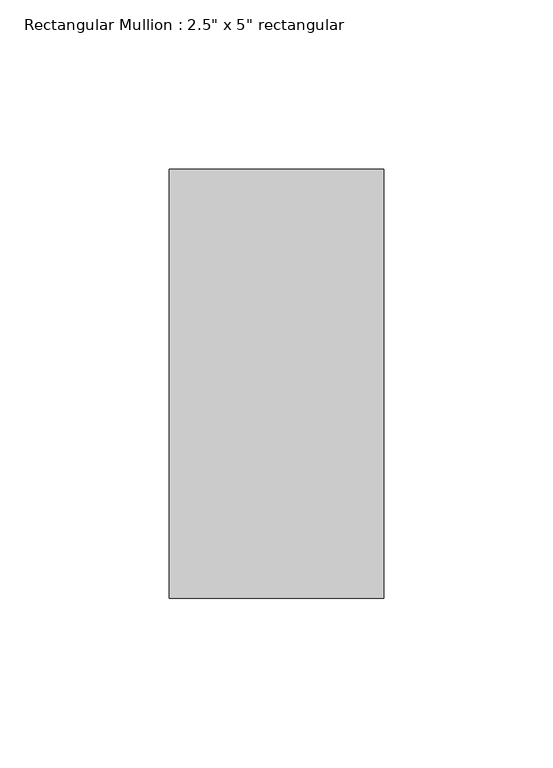
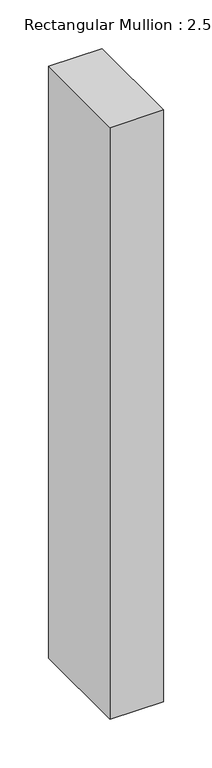
"""IFC4 building model written with IfcOpenShell, lengths in millimetres: member geometry."""

from ifc_helpers import new_model, si_unit, frame, origin, place, context, project, spatial, polyline, outline, extrude, source, transform, mapped, element, save


def member_3a0a7659(model_context):
    return source(origin(), model_context, "Body", "SweptSolid", [
        extrude(outline(polyline([(0.0, 63.5), (0.0, -63.5), (-63.5, -63.5), (-63.5, 63.5), (0.0, 63.5)])), frame((0.0, 0.0, -742.95), z_axis=(0.0, 0.0, 1.0), x_axis=(1.0, 0.0, 0.0)), (0.0, 0.0, 1.0), 742.95),
    ])


if __name__ == "__main__":
    model = new_model("IFC4")
    model_context = context("Model", 3, world=origin())
    ifc_project = project(units=[si_unit("LENGTHUNIT", "METRE", prefix="MILLI")], contexts=[model_context])
    site = spatial("IfcSite", under=ifc_project)
    building = spatial("IfcBuilding", under=site)
    placement = place(None, origin())
    member_shape = member_3a0a7659(model_context)
    element("IfcMember", 1, ObjectType="Rectangular Mullion : 2.5\" x 5\" rectangular", at=placement, inside=building, context=model_context, shape_type="MappedRepresentation", body=[
        mapped(member_shape, transform((0.0, 0.0, 0.0), x_axis=(1.0, 0.0, 0.0), y_axis=(0.0, 1.0, 0.0), z_axis=(0.0, 0.0, 1.0))),
    ])
    save(model, "model.ifc")

# Revit data of these elements
# Type "Rectangular Mullion : 2.5\" x 5\" rectangular"
#   built-in parameter 1007304 = 0.416667 (stored number, unit not read)
#   built-in parameter 1007301 = 0.104167 (stored number, unit not read)
#   built-in parameter 1007300 = 0.104167 (stored number, unit not read)
# Element 1 (IfcMember, "Rectangular Mullion : 2.5\" x 5\" rectangular")
#   Materials on its faces: "Aluminum"
# Materials
#   "Aluminum": class "Metal", colour RGB 247 247 247, transparency 0, Description = "Aluminum 6061", Cost = 0
